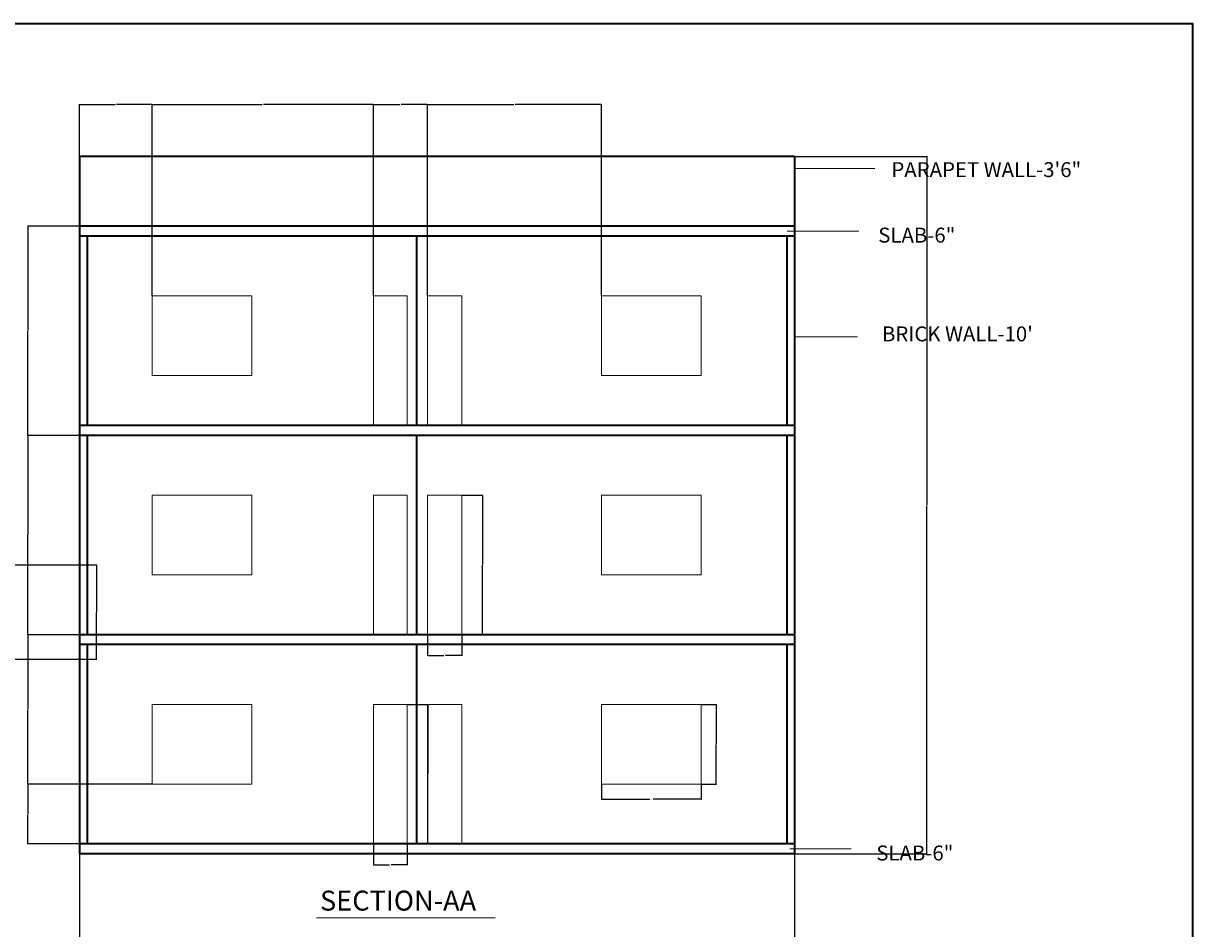
# Model space of a CAD drawing. Units: inches. Extents: x 992 to 2287, y 1476 to 2866.
# Tile 9 of 9: x 1583 to 2287, y 2321 to 2866. Entities that reach past the tile are written whole.
import ezdxf

# ---------------------------------------------------------------- set-up
doc = ezdxf.new("R2010")
doc.units = ezdxf.units.IN
for name, color, linetype, lineweight in [('A-ANNO-DIMS', 2, 'Continuous', 18), ('A-ANNO-TEXT', 7, 'Continuous', 18), ('A-ANNO-TTLB', 7, 'Continuous', 35), ('A-DOOR', 3, 'Continuous', 18), ('A-GLAZ', 4, 'Continuous', 18), ('A-SECT', 7, 'Continuous', 35)]:
    doc.layers.add(name, color=color, linetype=linetype, lineweight=lineweight)
doc.styles.get("Standard").update_dxf_attribs({"font": 'arial.ttf'})
doc.dimstyles.get("Standard").update_dxf_attribs({"dimtxt": 0.18, "dimasz": 0.18, "dimexe": 0.18, "dimexo": 0.0625, "dimgap": 0.09, "dimtad": 0, "dimtih": 1, "dimtoh": 1, "dimdec": 4, "dimzin": 0, "dimdsep": 46, "dimtxsty": 'Standard', "dimcen": 0.09, "dimadec": 0, "dimazin": 0, "dimtfac": 1, "dimtdec": 4, "dimtofl": 0, "dimtmove": 0, "dimatfit": 3, "dimfxl": 1, "dimtolj": 1, "dimtzin": 0, "dimarcsym": 0})

# ---------------------------------------------------------------- blocks, each defined once
blk = doc.blocks.new('WINDOW-SECTION-60X48')
for p, q in [((0, 48), (0, 0)), ((60, 48), (0, 48)), ((60, 48), (60, 0)), ((60, 0), (0, 0))]:
    blk.add_line(p, q)
blk = doc.blocks.new('DOOR-SECTION-84IN-A')
for p, q in [((0, 84), (0, 0)), ((20.2, 84), (0, 84)), ((20.2, 84), (20.2, 0)), ((20.2, 84), (20.2, 0))]:
    blk.add_line(p, q)
blk = doc.blocks.new('DOOR-SECTION-84IN-B')
for p, q in [((0, 84), (0, 0)), ((0, 84), (0, 0)), ((20.6, 84), (0, 84)), ((20.6, 84), (20.6, 0))]:
    blk.add_line(p, q)
blk = doc.blocks.new('*D94')
at = {"layer": 'A-ANNO-DIMS', "color": 0, "lineweight": -2, "transparency": 16777216}
for p, q in [((1555.36, 2540.13), (1627.25, 2540.13)), ((1627.07, 2539.95), (1627.07, 2511.94)), ((1627.07, 2483.58), (1627.07, 2511.58)), ((1555.36, 2483.4), (1627.25, 2483.4))]:
    blk.add_line(p, q, dxfattribs=at)
at = {"layer": 'A-ANNO-DIMS', "color": 0, "transparency": 16777216}
for points in [[(1627.04, 2539.95), (1627.1, 2539.95), (1627.07, 2540.13)], [(1627.04, 2483.58), (1627.1, 2483.58), (1627.07, 2483.4)]]:
    blk.add_solid(points, dxfattribs=at)
at = {"layer": 'Defpoints', "color": 0, "transparency": 16777216}
for p in [(1555.29, 2540.13), (1627.07, 2540.13), (1555.29, 2483.4)]:
    blk.add_point(p, dxfattribs=at)
at = {"layer": 'A-ANNO-DIMS', "color": 0, "transparency": 16777216, "insert": (1627.07, 2511.76), "char_height": 0.18, "attachment_point": 5}
blk.add_mtext('\\A1;57 TYP.', dxfattribs=at)
blk = doc.blocks.new('*D103')
at = {"layer": 'A-ANNO-DIMS', "color": 0, "lineweight": -2, "transparency": 16777216}
for p, q in [((1931.22, 2408.07), (1931.22, 2398.95)), ((1991.22, 2408.07), (1991.22, 2398.95)), ((1931.4, 2399.13), (1960.1, 2399.13)), ((1991.04, 2399.13), (1962.34, 2399.13))]:
    blk.add_line(p, q, dxfattribs=at)
at = {"layer": 'A-ANNO-DIMS', "color": 0, "transparency": 16777216}
for points in [[(1931.4, 2399.16), (1931.4, 2399.1), (1931.22, 2399.13)], [(1991.04, 2399.16), (1991.04, 2399.1), (1991.22, 2399.13)]]:
    blk.add_solid(points, dxfattribs=at)
at = {"layer": 'Defpoints', "color": 0, "transparency": 16777216}
for p in [(1931.22, 2408.13), (1991.22, 2408.13), (1991.22, 2399.13)]:
    blk.add_point(p, dxfattribs=at)
at = {"layer": 'A-ANNO-DIMS', "color": 0, "transparency": 16777216, "insert": (1961.22, 2399.13), "char_height": 0.18, "attachment_point": 5}
blk.add_mtext('\\A1;WINDOW 60 TYP.', dxfattribs=at)
blk = doc.blocks.new('*D104')
at = {"layer": 'A-ANNO-DIMS', "color": 0, "lineweight": -2, "transparency": 16777216}
for p, q in [((1991.29, 2456.13), (2000.4, 2456.13)), ((2000.22, 2455.95), (2000.22, 2432.31)), ((2000.22, 2408.31), (2000.22, 2431.95)), ((1991.29, 2408.13), (2000.4, 2408.13))]:
    blk.add_line(p, q, dxfattribs=at)
at = {"layer": 'A-ANNO-DIMS', "color": 0, "transparency": 16777216}
for points in [[(2000.19, 2455.95), (2000.25, 2455.95), (2000.22, 2456.13)], [(2000.19, 2408.31), (2000.25, 2408.31), (2000.22, 2408.13)]]:
    blk.add_solid(points, dxfattribs=at)
at = {"layer": 'Defpoints', "color": 0, "transparency": 16777216}
for p in [(1991.22, 2456.13), (2000.22, 2456.13), (1991.22, 2408.13)]:
    blk.add_point(p, dxfattribs=at)
at = {"layer": 'A-ANNO-DIMS', "color": 0, "transparency": 16777216, "insert": (2000.22, 2432.13), "char_height": 0.18, "attachment_point": 5}
blk.add_mtext('\\A1;48 TYP.', dxfattribs=at)
blk = doc.blocks.new('*D105')
at = {"layer": 'A-ANNO-DIMS', "color": 0, "lineweight": -2, "transparency": 16777216}
for p, q in [((1814.16, 2456.13), (1826.87, 2456.13)), ((1826.69, 2455.95), (1826.69, 2414.31)), ((1826.69, 2372.31), (1826.69, 2413.95)), ((1814.16, 2372.13), (1826.87, 2372.13))]:
    blk.add_line(p, q, dxfattribs=at)
at = {"layer": 'A-ANNO-DIMS', "color": 0, "transparency": 16777216}
for points in [[(1826.66, 2455.95), (1826.72, 2455.95), (1826.69, 2456.13)], [(1826.66, 2372.31), (1826.72, 2372.31), (1826.69, 2372.13)]]:
    blk.add_solid(points, dxfattribs=at)
at = {"layer": 'Defpoints', "color": 0, "transparency": 16777216}
for p in [(1814.09, 2456.13), (1826.69, 2456.13), (1814.09, 2372.13)]:
    blk.add_point(p, dxfattribs=at)
at = {"layer": 'A-ANNO-DIMS', "color": 0, "transparency": 16777216, "insert": (1826.69, 2414.13), "char_height": 0.18, "attachment_point": 5}
blk.add_mtext('\\A1;DOOR 84 TYP.', dxfattribs=at)
blk = doc.blocks.new('*D106')
at = {"layer": 'A-ANNO-DIMS', "color": 0, "lineweight": -2, "transparency": 16777216}
for p, q in [((1793.89, 2372.07), (1793.89, 2359.35)), ((1814.09, 2372.07), (1814.09, 2359.35)), ((1794.07, 2359.53), (1803.46, 2359.53)), ((1813.91, 2359.53), (1804.52, 2359.53))]:
    blk.add_line(p, q, dxfattribs=at)
at = {"layer": 'A-ANNO-DIMS', "color": 0, "transparency": 16777216}
for points in [[(1794.07, 2359.56), (1794.07, 2359.5), (1793.89, 2359.53)], [(1813.91, 2359.56), (1813.91, 2359.5), (1814.09, 2359.53)]]:
    blk.add_solid(points, dxfattribs=at)
at = {"layer": 'Defpoints', "color": 0, "transparency": 16777216}
for p in [(1793.89, 2372.13), (1814.09, 2372.13), (1814.09, 2359.53)]:
    blk.add_point(p, dxfattribs=at)
at = {"layer": 'A-ANNO-DIMS', "color": 0, "transparency": 16777216, "insert": (1803.99, 2359.53), "char_height": 0.18, "attachment_point": 5}
blk.add_mtext('\\A1;20 TYP.', dxfattribs=at)
blk = doc.blocks.new('*D107')
at = {"layer": 'A-ANNO-DIMS', "color": 0, "lineweight": -2, "transparency": 16777216}
for p, q in [((1847.09, 2582.13), (1859.81, 2582.13)), ((1859.63, 2581.95), (1859.63, 2540.31)), ((1859.63, 2498.31), (1859.63, 2539.95)), ((1847.09, 2498.13), (1859.81, 2498.13))]:
    blk.add_line(p, q, dxfattribs=at)
at = {"layer": 'A-ANNO-DIMS', "color": 0, "transparency": 16777216}
for points in [[(1859.6, 2581.95), (1859.66, 2581.95), (1859.63, 2582.13)], [(1859.6, 2498.31), (1859.66, 2498.31), (1859.63, 2498.13)]]:
    blk.add_solid(points, dxfattribs=at)
at = {"layer": 'Defpoints', "color": 0, "transparency": 16777216}
for p in [(1847.03, 2582.13), (1859.63, 2582.13), (1847.03, 2498.13)]:
    blk.add_point(p, dxfattribs=at)
at = {"layer": 'A-ANNO-DIMS', "color": 0, "transparency": 16777216, "insert": (1859.63, 2540.13), "char_height": 0.18, "attachment_point": 5}
blk.add_mtext('\\A1;DOOR 84 TYP.', dxfattribs=at)
blk = doc.blocks.new('*D108')
at = {"layer": 'A-ANNO-DIMS', "color": 0, "lineweight": -2, "transparency": 16777216}
for p, q in [((1826.43, 2498.07), (1826.43, 2485.35)), ((1847.03, 2498.07), (1847.03, 2485.35)), ((1826.61, 2485.53), (1836.2, 2485.53)), ((1846.85, 2485.53), (1837.26, 2485.53))]:
    blk.add_line(p, q, dxfattribs=at)
at = {"layer": 'A-ANNO-DIMS', "color": 0, "transparency": 16777216}
for points in [[(1826.61, 2485.56), (1826.61, 2485.5), (1826.43, 2485.53)], [(1846.85, 2485.56), (1846.85, 2485.5), (1847.03, 2485.53)]]:
    blk.add_solid(points, dxfattribs=at)
at = {"layer": 'Defpoints', "color": 0, "transparency": 16777216}
for p in [(1826.43, 2498.13), (1847.03, 2498.13), (1847.03, 2485.53)]:
    blk.add_point(p, dxfattribs=at)
at = {"layer": 'A-ANNO-DIMS', "color": 0, "transparency": 16777216, "insert": (1836.73, 2485.53), "char_height": 0.18, "attachment_point": 5}
blk.add_mtext('\\A1;21 TYP.', dxfattribs=at)
blk = doc.blocks.new('*D141')
at = {"layer": 'A-ANNO-DIMS', "color": 0, "lineweight": -2, "transparency": 16777216}
for p, q in [((2047.46, 2786.13), (2127.25, 2786.13)), ((2127.07, 2785.95), (2127.07, 2576.31)), ((2127.07, 2366.31), (2127.07, 2575.95)), ((2047.46, 2366.13), (2127.25, 2366.13))]:
    blk.add_line(p, q, dxfattribs=at)
at = {"layer": 'A-ANNO-DIMS', "color": 0, "transparency": 16777216}
for points in [[(2127.04, 2785.95), (2127.1, 2785.95), (2127.07, 2786.13)], [(2127.04, 2366.31), (2127.1, 2366.31), (2127.07, 2366.13)]]:
    blk.add_solid(points, dxfattribs=at)
at = {"layer": 'Defpoints', "color": 0, "transparency": 16777216}
for p in [(2047.39, 2786.13), (2127.07, 2786.13), (2047.39, 2366.13)]:
    blk.add_point(p, dxfattribs=at)
at = {"layer": 'A-ANNO-DIMS', "color": 0, "transparency": 16777216, "insert": (2127.07, 2576.13), "char_height": 0.18, "attachment_point": 5}
blk.add_mtext('\\A1;420', dxfattribs=at)
blk = doc.blocks.new('*D142')
at = {"layer": 'A-ANNO-DIMS', "color": 0, "lineweight": -2, "transparency": 16777216}
for p, q in [((1616.89, 2366.07), (1616.89, 2296.22)), ((2047.39, 2366.07), (2047.39, 2296.22)), ((1617.07, 2296.4), (1831.75, 2296.4)), ((2047.21, 2296.4), (1832.54, 2296.4))]:
    blk.add_line(p, q, dxfattribs=at)
at = {"layer": 'A-ANNO-DIMS', "color": 0, "transparency": 16777216}
for points in [[(1617.07, 2296.43), (1617.07, 2296.37), (1616.89, 2296.4)], [(2047.21, 2296.43), (2047.21, 2296.37), (2047.39, 2296.4)]]:
    blk.add_solid(points, dxfattribs=at)
at = {"layer": 'Defpoints', "color": 0, "transparency": 16777216}
for p in [(1616.89, 2366.13), (2047.39, 2366.13), (2047.39, 2296.4)]:
    blk.add_point(p, dxfattribs=at)
at = {"layer": 'A-ANNO-DIMS', "color": 0, "transparency": 16777216, "insert": (1832.14, 2296.4), "char_height": 0.18, "attachment_point": 5}
blk.add_mtext('\\A1;430.5', dxfattribs=at)
blk = doc.blocks.new('*D143')
at = {"layer": 'A-ANNO-DIMS', "color": 0, "lineweight": -2, "transparency": 16777216}
for p, q in [((1616.89, 2786.19), (1616.89, 2817.51)), ((1617.07, 2817.33), (1638.38, 2817.33)), ((1660.47, 2817.33), (1639.17, 2817.33)), ((1660.65, 2702.19), (1660.65, 2817.51))]:
    blk.add_line(p, q, dxfattribs=at)
at = {"layer": 'A-ANNO-DIMS', "color": 0, "transparency": 16777216}
for points in [[(1617.07, 2817.36), (1617.07, 2817.3), (1616.89, 2817.33)], [(1660.47, 2817.36), (1660.47, 2817.3), (1660.65, 2817.33)]]:
    blk.add_solid(points, dxfattribs=at)
at = {"layer": 'Defpoints', "color": 0, "transparency": 16777216}
for p in [(1660.65, 2817.33), (1616.89, 2786.13), (1660.65, 2702.13)]:
    blk.add_point(p, dxfattribs=at)
at = {"layer": 'A-ANNO-DIMS', "color": 0, "transparency": 16777216, "insert": (1638.77, 2817.33), "char_height": 0.18, "attachment_point": 5}
blk.add_mtext('\\A1;43.76', dxfattribs=at)
blk = doc.blocks.new('*D144')
at = {"layer": 'A-ANNO-DIMS', "color": 0, "lineweight": -2, "transparency": 16777216}
for p, q in [((1660.65, 2702.19), (1660.65, 2817.51)), ((1660.83, 2817.33), (1726.82, 2817.33)), ((1793.71, 2817.33), (1727.73, 2817.33)), ((1793.89, 2702.19), (1793.89, 2817.51))]:
    blk.add_line(p, q, dxfattribs=at)
at = {"layer": 'A-ANNO-DIMS', "color": 0, "transparency": 16777216}
for points in [[(1660.83, 2817.36), (1660.83, 2817.3), (1660.65, 2817.33)], [(1793.71, 2817.36), (1793.71, 2817.3), (1793.89, 2817.33)]]:
    blk.add_solid(points, dxfattribs=at)
at = {"layer": 'Defpoints', "color": 0, "transparency": 16777216}
for p in [(1793.89, 2817.33), (1660.65, 2702.13), (1793.89, 2702.13)]:
    blk.add_point(p, dxfattribs=at)
at = {"layer": 'A-ANNO-DIMS', "color": 0, "transparency": 16777216, "insert": (1727.27, 2817.33), "char_height": 0.18, "attachment_point": 5}
blk.add_mtext('\\A1;133.24', dxfattribs=at)
blk = doc.blocks.new('*D145')
at = {"layer": 'A-ANNO-DIMS', "color": 0, "lineweight": -2, "transparency": 16777216}
for p, q in [((1793.89, 2702.19), (1793.89, 2817.51)), ((1794.07, 2817.33), (1809.77, 2817.33)), ((1826.25, 2817.33), (1810.56, 2817.33)), ((1826.43, 2702.19), (1826.43, 2817.51))]:
    blk.add_line(p, q, dxfattribs=at)
at = {"layer": 'A-ANNO-DIMS', "color": 0, "transparency": 16777216}
for points in [[(1794.07, 2817.36), (1794.07, 2817.3), (1793.89, 2817.33)], [(1826.25, 2817.36), (1826.25, 2817.3), (1826.43, 2817.33)]]:
    blk.add_solid(points, dxfattribs=at)
at = {"layer": 'Defpoints', "color": 0, "transparency": 16777216}
for p in [(1826.43, 2817.33), (1793.89, 2702.13), (1826.43, 2702.13)]:
    blk.add_point(p, dxfattribs=at)
at = {"layer": 'A-ANNO-DIMS', "color": 0, "transparency": 16777216, "insert": (1810.16, 2817.33), "char_height": 0.18, "attachment_point": 5}
blk.add_mtext('\\A1;32.54', dxfattribs=at)
blk = doc.blocks.new('*D146')
at = {"layer": 'A-ANNO-DIMS', "color": 0, "lineweight": -2, "transparency": 16777216}
for p, q in [((1826.43, 2702.19), (1826.43, 2817.51)), ((1826.61, 2817.33), (1878.44, 2817.33)), ((1931.04, 2817.33), (1879.21, 2817.33)), ((1931.22, 2702.19), (1931.22, 2817.51))]:
    blk.add_line(p, q, dxfattribs=at)
at = {"layer": 'A-ANNO-DIMS', "color": 0, "transparency": 16777216}
for points in [[(1826.61, 2817.36), (1826.61, 2817.3), (1826.43, 2817.33)], [(1931.04, 2817.36), (1931.04, 2817.3), (1931.22, 2817.33)]]:
    blk.add_solid(points, dxfattribs=at)
at = {"layer": 'Defpoints', "color": 0, "transparency": 16777216}
for p in [(1931.22, 2817.33), (1826.43, 2702.13), (1931.22, 2702.13)]:
    blk.add_point(p, dxfattribs=at)
at = {"layer": 'A-ANNO-DIMS', "color": 0, "transparency": 16777216, "insert": (1878.83, 2817.33), "char_height": 0.18, "attachment_point": 5}
blk.add_mtext('\\A1;104.8', dxfattribs=at)
blk = doc.blocks.new('*D147')
at = {"layer": 'A-ANNO-DIMS', "color": 0, "lineweight": -2, "transparency": 16777216}
for p, q in [((1660.59, 2408.13), (1585.51, 2408.13)), ((1585.69, 2407.95), (1585.69, 2390.31)), ((1585.69, 2372.31), (1585.69, 2389.95)), ((1616.83, 2372.13), (1585.51, 2372.13))]:
    blk.add_line(p, q, dxfattribs=at)
at = {"layer": 'A-ANNO-DIMS', "color": 0, "transparency": 16777216}
for points in [[(1585.66, 2407.95), (1585.72, 2407.95), (1585.69, 2408.13)], [(1585.66, 2372.31), (1585.72, 2372.31), (1585.69, 2372.13)]]:
    blk.add_solid(points, dxfattribs=at)
at = {"layer": 'Defpoints', "color": 0, "transparency": 16777216}
for p in [(1585.69, 2408.13), (1660.65, 2408.13), (1616.89, 2372.13)]:
    blk.add_point(p, dxfattribs=at)
at = {"layer": 'A-ANNO-DIMS', "color": 0, "transparency": 16777216, "insert": (1585.69, 2390.13), "char_height": 0.18, "attachment_point": 5}
blk.add_mtext('\\A1;36', dxfattribs=at)
blk = doc.blocks.new('*D148')
at = {"layer": 'A-ANNO-DIMS', "color": 0, "lineweight": -2, "transparency": 16777216}
for p, q in [((1616.83, 2498.13), (1585.51, 2498.13)), ((1585.69, 2497.95), (1585.69, 2453.31)), ((1585.69, 2408.31), (1585.69, 2452.95)), ((1660.59, 2408.13), (1585.51, 2408.13))]:
    blk.add_line(p, q, dxfattribs=at)
at = {"layer": 'A-ANNO-DIMS', "color": 0, "transparency": 16777216}
for points in [[(1585.66, 2497.95), (1585.72, 2497.95), (1585.69, 2498.13)], [(1585.66, 2408.31), (1585.72, 2408.31), (1585.69, 2408.13)]]:
    blk.add_solid(points, dxfattribs=at)
at = {"layer": 'Defpoints', "color": 0, "transparency": 16777216}
for p in [(1585.69, 2498.13), (1616.89, 2498.13), (1660.65, 2408.13)]:
    blk.add_point(p, dxfattribs=at)
at = {"layer": 'A-ANNO-DIMS', "color": 0, "transparency": 16777216, "insert": (1585.69, 2453.13), "char_height": 0.18, "attachment_point": 5}
blk.add_mtext('\\A1;90', dxfattribs=at)
blk = doc.blocks.new('*D149')
at = {"layer": 'A-ANNO-DIMS', "color": 0, "lineweight": -2, "transparency": 16777216}
for p, q in [((1616.83, 2744.13), (1585.51, 2744.13)), ((1585.69, 2743.95), (1585.69, 2681.31)), ((1585.69, 2618.31), (1585.69, 2680.95)), ((1616.83, 2618.13), (1585.51, 2618.13))]:
    blk.add_line(p, q, dxfattribs=at)
at = {"layer": 'A-ANNO-DIMS', "color": 0, "transparency": 16777216}
for points in [[(1585.66, 2743.95), (1585.72, 2743.95), (1585.69, 2744.13)], [(1585.66, 2618.31), (1585.72, 2618.31), (1585.69, 2618.13)]]:
    blk.add_solid(points, dxfattribs=at)
at = {"layer": 'Defpoints', "color": 0, "transparency": 16777216}
for p in [(1585.69, 2744.13), (1616.89, 2744.13), (1616.89, 2618.13)]:
    blk.add_point(p, dxfattribs=at)
at = {"layer": 'A-ANNO-DIMS', "color": 0, "transparency": 16777216, "insert": (1585.69, 2681.13), "char_height": 0.18, "attachment_point": 5}
blk.add_mtext('\\A1;126', dxfattribs=at)
blk = doc.blocks.new('*D150')
at = {"layer": 'A-ANNO-DIMS', "color": 0, "lineweight": -2, "transparency": 16777216}
for p, q in [((1616.83, 2618.13), (1585.51, 2618.13)), ((1585.69, 2617.95), (1585.69, 2558.31)), ((1585.69, 2498.31), (1585.69, 2557.95)), ((1616.83, 2498.13), (1585.51, 2498.13))]:
    blk.add_line(p, q, dxfattribs=at)
at = {"layer": 'A-ANNO-DIMS', "color": 0, "transparency": 16777216}
for points in [[(1585.66, 2617.95), (1585.72, 2617.95), (1585.69, 2618.13)], [(1585.66, 2498.31), (1585.72, 2498.31), (1585.69, 2498.13)]]:
    blk.add_solid(points, dxfattribs=at)
at = {"layer": 'Defpoints', "color": 0, "transparency": 16777216}
for p in [(1585.69, 2618.13), (1616.89, 2618.13), (1616.89, 2498.13)]:
    blk.add_point(p, dxfattribs=at)
at = {"layer": 'A-ANNO-DIMS', "color": 0, "transparency": 16777216, "insert": (1585.69, 2558.13), "char_height": 0.18, "attachment_point": 5}
blk.add_mtext('\\A1;120', dxfattribs=at)

msp = doc.modelspace()

# ---------------------------------------------------------------- linework, layer by layer
at = {"layer": 'A-ANNO-TEXT'}
for p, q in [((2047.3946, 2778.8765), (2095.8724, 2778.8765)), ((2043.1063, 2741.1051), (2086.2727, 2741.1051)), ((2047.3946, 2677.41), (2085.3659, 2677.41)), ((2044.677, 2369.2185), (2081.6, 2369.2185)), ((1759.5125, 2327.6015), (1867.0856, 2327.6015))]:
    msp.add_line(p, q, dxfattribs=at)
at = {"layer": 'A-ANNO-TTLB'}
msp.add_lwpolyline([(992.3484, 2866.1952), (2287.217, 2866.1952), (2287.217, 1476.4066), (992.3484, 1476.4066)], close=True, dxfattribs=at)
at = {"layer": 'A-DOOR'}
for p, q in [((1793.8946, 2702.1302), (1793.8946, 2624.1302)), ((1814.0937, 2702.1302), (1793.8946, 2702.1302)), ((1814.0937, 2702.1302), (1814.0937, 2624.1302)), ((1814.0937, 2702.1302), (1814.0937, 2624.1302)), ((1826.4319, 2702.1302), (1826.4319, 2624.1302)), ((1826.4319, 2702.1302), (1826.4319, 2624.1302)), ((1847.0287, 2702.1302), (1826.4319, 2702.1302)), ((1847.0287, 2702.1302), (1847.0287, 2624.1302))]:
    msp.add_line(p, q, dxfattribs=at)
at = {"layer": 'A-SECT'}
for p, q in [((1616.8946, 2786.1302), (1616.8946, 2612.1302)), ((2047.3946, 2786.1302), (1616.8946, 2786.1302)), ((2047.3946, 2786.1302), (2047.3946, 2612.1302)), ((2047.3946, 2744.1302), (1616.8946, 2744.1302)), ((2047.3946, 2738.1302), (1616.8946, 2738.1302)), ((1621.3946, 2738.1302), (1621.3946, 2624.1302)), ((1820.0284, 2624.1302), (1820.0284, 2738.1302)), ((2042.8946, 2738.1302), (2042.8946, 2624.1302)), ((1616.8946, 2666.1302), (1616.8946, 2492.1302)), ((2047.3946, 2666.1302), (2047.3946, 2492.1302)), ((2047.3946, 2624.1302), (1616.8946, 2624.1302)), ((2047.3946, 2618.1302), (1616.8946, 2618.1302)), ((1621.3946, 2618.1302), (1621.3946, 2498.1302)), ((1820.0284, 2498.1302), (1820.0284, 2618.1302)), ((2042.8946, 2618.1302), (2042.8946, 2498.1302)), ((1616.8946, 2540.1302), (1616.8946, 2366.1302)), ((2047.3946, 2540.1302), (2047.3946, 2366.1302)), ((2047.3946, 2498.1302), (1616.8946, 2498.1302)), ((2047.3946, 2492.1302), (1616.8946, 2492.1302)), ((1621.3946, 2492.1302), (1621.3946, 2372.1302)), ((1820.0284, 2372.1302), (1820.0284, 2492.1302)), ((2042.8946, 2492.1302), (2042.8946, 2372.1302)), ((2047.3946, 2372.1302), (1616.8946, 2372.1302)), ((2047.3946, 2366.1302), (1616.8946, 2366.1302))]:
    msp.add_line(p, q, dxfattribs=at)

# ---------------------------------------------------------------- block references
at = {"layer": 'A-DOOR'}
for name, p in [('DOOR-SECTION-84IN-A', (1793.895, 2498.13)), ('DOOR-SECTION-84IN-B', (1826.432, 2498.13)), ('DOOR-SECTION-84IN-A', (1793.895, 2372.13)), ('DOOR-SECTION-84IN-B', (1826.432, 2372.13))]:
    msp.add_blockref(name, p, dxfattribs=at)
at = {"layer": 'A-GLAZ'}
for p in [(1660.655, 2654.13), (1931.2234, 2654.13), (1660.655, 2534.13), (1931.2234, 2534.13), (1660.655, 2408.13), (1931.2234, 2408.13)]:
    msp.add_blockref('WINDOW-SECTION-60X48', p, dxfattribs=at)

# ---------------------------------------------------------------- texts
at = {"layer": 'A-ANNO-TEXT', "attachment_point": 1}
for s, width, insert, char_height in [('PARAPET WALL-3\'6"', 210.567118, (2105.7992, 2782.6324), 9), ('SLAB-6"', 49.863332, (2097.8952, 2743.1966), 9), ("BRICK WALL-10'", 111.223695, (2100.138, 2683.7274), 9), ('SLAB-6"', 65.06107, (2096.701, 2371.1749), 9), ('SECTION-AA', 200.536665, (1761.6867, 2343.9872), 12)]:
    msp.add_mtext_dynamic_manual_height_columns(s, width=width, gutter_width=12.5, heights=[0], dxfattribs=dict(at, insert=insert, char_height=char_height))

# ---------------------------------------------------------------- dimensions: what is measured, and where the dimension line sits
at = {"layer": 'A-ANNO-DIMS'}
for base, p1, p2, override, picture, middle in [((1660.6549, 2817.3302), (1616.8946, 2786.1302), (1660.6549, 2702.1302), {"dimdec": 2, "dimlfac": 1, "dimrnd": 0, "dimzin": 0, "dimdsep": 46, "dimlunit": 2}, '*D143', (1638.7747, 2817.3302)), ((1793.8946, 2817.3302), (1660.6549, 2702.1302), (1793.8946, 2702.1302), {"dimdec": 2, "dimlfac": 1, "dimrnd": 0, "dimzin": 0, "dimdsep": 46, "dimlunit": 2}, '*D144', (1727.2747, 2817.3302)), ((1826.4319, 2817.3302), (1793.8946, 2702.1302), (1826.4319, 2702.1302), {"dimdec": 2, "dimlfac": 1, "dimrnd": 0, "dimzin": 0, "dimdsep": 46, "dimlunit": 2}, '*D145', (1810.1632, 2817.3302)), ((1931.2233, 2817.3302), (1826.4319, 2702.1302), (1931.2233, 2702.1302), {"dimdec": 1, "dimlfac": 1, "dimrnd": 0, "dimzin": 0, "dimdsep": 46, "dimlunit": 2}, '*D146', (1878.8276, 2817.3302)), ((2047.3946, 2296.4015), (1616.8946, 2366.1302), (2047.3946, 2366.1302), {"dimdec": 1, "dimlfac": 1, "dimrnd": 0, "dimzin": 0, "dimdsep": 46, "dimlunit": 2}, '*D142', (1832.1446, 2296.4015))]:
    dim = msp.add_linear_dim(base=base, p1=p1, p2=p2, dimstyle='Standard', override=override, dxfattribs=at)
    dim.commit()
    dim.dimension.update_dxf_attribs({"geometry": picture, "text_midpoint": middle})
for base, p1, p2, picture, middle in [((2127.0724, 2786.1302), (2047.3946, 2366.1302), (2047.3946, 2786.1302), '*D141', (2127.0724, 2576.1302)), ((1585.6946, 2744.1302), (1616.8946, 2618.1302), (1616.8946, 2744.1302), '*D149', (1585.6946, 2681.1302)), ((1585.6946, 2618.1302), (1616.8946, 2498.1302), (1616.8946, 2618.1302), '*D150', (1585.6946, 2558.1302)), ((1585.6946, 2498.1302), (1660.6549, 2408.1302), (1616.8946, 2498.1302), '*D148', (1585.6946, 2453.1302)), ((1585.6946, 2408.1302), (1616.8946, 2372.1302), (1660.6549, 2408.1302), '*D147', (1585.6946, 2390.1302))]:
    dim = msp.add_linear_dim(base=base, p1=p1, p2=p2, angle=90, dimstyle='Standard', override={"dimdec": 0, "dimlfac": 1, "dimrnd": 0, "dimzin": 0, "dimdsep": 46, "dimlunit": 2}, dxfattribs=at)
    dim.commit()
    dim.dimension.update_dxf_attribs({"geometry": picture, "text_midpoint": middle})
for base, p1, p2, text, picture, middle in [((1859.6287, 2582.1302), (1847.0287, 2498.1302), (1847.0287, 2582.1302), 'DOOR <> TYP.', '*D107', (1859.6287, 2540.1302)), ((1627.0686, 2540.1302), (1555.2936, 2483.396), (1555.2936, 2540.1302), '<> TYP.', '*D94', (1627.0686, 2511.7631)), ((1826.6937, 2456.1302), (1814.0937, 2372.1302), (1814.0937, 2456.1302), 'DOOR <> TYP.', '*D105', (1826.6937, 2414.1302)), ((2000.2233, 2456.1302), (1991.2233, 2408.1302), (1991.2233, 2456.1302), '<> TYP.', '*D104', (2000.2233, 2432.1302))]:
    dim = msp.add_linear_dim(base=base, p1=p1, p2=p2, angle=90, text=text, dimstyle='Standard', override={"dimdec": 0, "dimlfac": 1, "dimrnd": 0, "dimzin": 0, "dimdsep": 46, "dimlunit": 2}, dxfattribs=at)
    dim.commit()
    dim.dimension.update_dxf_attribs({"geometry": picture, "text_midpoint": middle})
for base, p1, p2, text, picture, middle in [((1847.0287, 2485.5302), (1826.4319, 2498.1302), (1847.0287, 2498.1302), '<> TYP.', '*D108', (1836.7303, 2485.5302)), ((1991.2233, 2399.1302), (1931.2233, 2408.1302), (1991.2233, 2408.1302), 'WINDOW <> TYP.', '*D103', (1961.2233, 2399.1302)), ((1814.0937, 2359.5302), (1793.8946, 2372.1302), (1814.0937, 2372.1302), '<> TYP.', '*D106', (1803.9941, 2359.5302))]:
    dim = msp.add_linear_dim(base=base, p1=p1, p2=p2, text=text, dimstyle='Standard', override={"dimdec": 0, "dimlfac": 1, "dimrnd": 0, "dimzin": 0, "dimdsep": 46, "dimlunit": 2}, dxfattribs=at)
    dim.commit()
    dim.dimension.update_dxf_attribs({"geometry": picture, "text_midpoint": middle})

doc.saveas('drawing.dxf')
